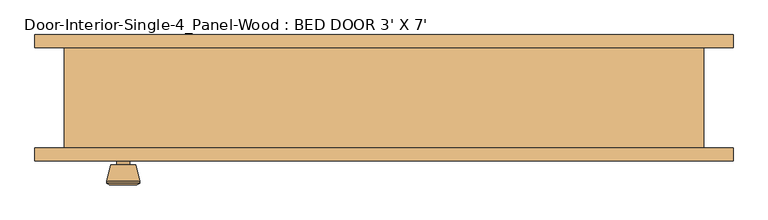
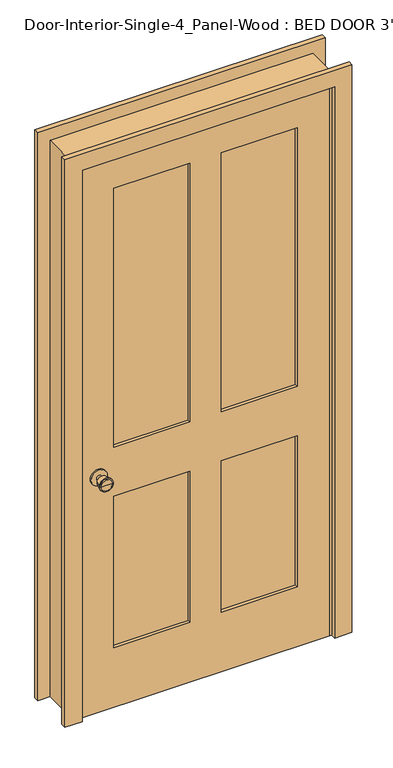
"""IFC4 building model written with IfcOpenShell, lengths in millimetres: door geometry, Door-Interior-Single-4_Panel-Wood : BED DOOR 3' X 7'."""

from ifc_helpers import new_model, si_unit, point, frame, frame_2d, origin, place, context, project, spatial, polyline, circle_curve, trimmed, segment, composite_curve, outline, extrude, faceted_brep, source, transform, mapped, element, save
from ifc_brep_helpers import plane_surface, cylinder_surface, revolved_surface, advanced_brep


def door_interior_single_4_panel_wood_bed_door_3_x_7_5a83478c(model_context):
    return source(origin(), model_context, "Body", "SolidModel", [
        advanced_brep(
        [(-393.7, -32.1, 914.4), (-403.7, -32.1, 914.4), (-383.7, -32.1, 914.4), (-373.2241324, 16.9, 914.4), (-414.1758676, 16.9, 914.4), (-393.7, 16.9, 914.4), (-368.7, 15.0721319, 914.4), (-418.7, 15.0721319, 914.4), (-368.7, 11.6084537, 914.4), (-418.7, 11.6084537, 914.4), (-375.063764, -13.1, 914.4), (-412.336236, -13.1, 914.4), (-383.7, -13.1, 914.4), (-403.7, -13.1, 914.4)],
        [
            (0, 1),
            (1, 2, circle_curve(frame((-393.7, -32.1, 914.4), z_axis=(0.0, -1.0, 0.0), x_axis=(-1.0, 0.0, 0.0)), 10.0)),
            (2, 0),
            (2, 1, circle_curve(frame((-393.7, -32.1, 914.4), z_axis=(0.0, -1.0, 0.0), x_axis=(-1.0, 0.0, 0.0)), 10.0)),
            (3, 4, circle_curve(frame((-393.7, 16.9, 914.4), z_axis=(0.0, 1.0, 0.0), x_axis=(-1.0, 0.0, 0.0)), 20.4758676)),
            (4, 5),
            (5, 3),
            (4, 3, circle_curve(frame((-393.7, 16.9, 914.4), z_axis=(0.0, 1.0, 0.0), x_axis=(-1.0, 0.0, 0.0)), 20.4758676)),
            (6, 7, circle_curve(frame((-393.7, 15.0721319, 914.4), z_axis=(0.0, 1.0, 0.0), x_axis=(-1.0, 0.0, 0.0)), 25.0)),
            (7, 4),
            (3, 6),
            (7, 6, circle_curve(frame((-393.7, 15.0721319, 914.4), z_axis=(0.0, 1.0, 0.0), x_axis=(-1.0, 0.0, 0.0)), 25.0)),
            (8, 9, circle_curve(frame((-393.7, 11.6084537, 914.4), z_axis=(0.0, 1.0, 0.0), x_axis=(-1.0, 0.0, 0.0)), 25.0)),
            (9, 7),
            (6, 8),
            (9, 8, circle_curve(frame((-393.7, 11.6084537, 914.4), z_axis=(0.0, 1.0, 0.0), x_axis=(-1.0, 0.0, 0.0)), 25.0)),
            (10, 11, circle_curve(frame((-393.7, -13.1, 914.4), z_axis=(0.0, 1.0, 0.0), x_axis=(-1.0, 0.0, 0.0)), 18.636236)),
            (11, 9),
            (8, 10),
            (11, 10, circle_curve(frame((-393.7, -13.1, 914.4), z_axis=(0.0, 1.0, 0.0), x_axis=(-1.0, 0.0, 0.0)), 18.636236)),
            (12, 13, circle_curve(frame((-393.7, -13.1, 914.4), z_axis=(0.0, 1.0, 0.0), x_axis=(-1.0, 0.0, 0.0)), 10.0)),
            (13, 11),
            (10, 12),
            (13, 12, circle_curve(frame((-393.7, -13.1, 914.4), z_axis=(0.0, 1.0, 0.0), x_axis=(-1.0, 0.0, 0.0)), 10.0)),
            (1, 13),
            (12, 2),
        ],
        [
            plane_surface(frame((-393.7, -32.1, 914.4), z_axis=(0.0, -1.0, 0.0), x_axis=(-1.0, 0.0, 0.0))),
            plane_surface(frame((-393.7, 16.9, 914.4), z_axis=(0.0, 1.0, 0.0), x_axis=(-1.0, 0.0, 0.0))),
            revolved_surface(polyline([(-414.1758676, 16.9, 914.4), (-418.7, 15.0721319, 914.4)]), (-393.7, -32.1, 914.4), (0.0, -1.0, 0.0)),
            cylinder_surface(frame((-393.7, -32.1, 914.4), z_axis=(0.0, -1.0, 0.0), x_axis=(-1.0, 0.0, 0.0)), 25.0),
            revolved_surface(polyline([(-418.7, 11.6084537, 914.4), (-412.336236, -13.1, 914.4)]), (-393.7, -32.1, 914.4), (0.0, -1.0, 0.0)),
            plane_surface(frame((-393.7, -13.1, 914.4), z_axis=(0.0, -1.0, 0.0), x_axis=(-1.0, 0.0, 0.0))),
            cylinder_surface(frame((-393.7, -32.1, 914.4), z_axis=(0.0, -1.0, 0.0), x_axis=(-1.0, 0.0, 0.0)), 10.0),
        ],
        [
            (0, [[1, 2, 3]]),
            (0, [[-3, 4, -1]]),
            (1, [[5, 6, 7]]),
            (1, [[8, -7, -6]]),
            (2, [[9, 10, -5, 11]]),
            (2, [[12, -11, -8, -10]]),
            (3, [[13, 14, -9, 15]]),
            (3, [[16, -15, -12, -14]]),
            (4, [[17, 18, -13, 19]]),
            (4, [[20, -19, -16, -18]]),
            (5, [[21, 22, -17, 23]]),
            (5, [[24, -23, -20, -22]]),
            (6, [[-2, 25, -21, 26]]),
            (6, [[-4, -26, -24, -25]]),
        ],
    ),
        extrude(outline(composite_curve([segment(trimmed(circle_curve(frame_2d((914.4, -393.7)), 30.0), [point((914.4, -423.7))], [point((914.4, -363.7))], False, "CARTESIAN"), True, "CONTINUOUS"), segment(trimmed(circle_curve(frame_2d((914.4, -393.7)), 30.0), [point((914.4, -363.7))], [point((914.4, -423.7))], False, "CARTESIAN"), True, "CONTINUOUS")], self_intersect=False)), frame((0.0, -38.1, 0.0), z_axis=(0.0, 1.0, 0.0), x_axis=(0.0, 0.0, 1.0)), (0.0, 0.0, 1.0), 6.0),
        advanced_brep(
        [(-393.7, -79.025, 914.4), (-383.7, -79.025, 914.4), (-403.7, -79.025, 914.4), (-373.2241324, -128.025, 914.4), (-393.7, -128.025, 914.4), (-414.1758676, -128.025, 914.4), (-368.7, -126.1971319, 914.4), (-418.7, -126.1971319, 914.4), (-368.7, -122.7334537, 914.4), (-418.7, -122.7334537, 914.4), (-375.063764, -98.025, 914.4), (-412.336236, -98.025, 914.4), (-383.7, -98.025, 914.4), (-403.7, -98.025, 914.4)],
        [
            (0, 1),
            (1, 2, circle_curve(frame((-393.7, -79.025, 914.4), z_axis=(0.0, 1.0, 0.0), x_axis=(-1.0, 0.0, 0.0)), 10.0)),
            (2, 0),
            (2, 1, circle_curve(frame((-393.7, -79.025, 914.4), z_axis=(0.0, 1.0, 0.0), x_axis=(-1.0, 0.0, 0.0)), 10.0)),
            (3, 4),
            (4, 5),
            (5, 3, circle_curve(frame((-393.7, -128.025, 914.4), z_axis=(0.0, -1.0, 0.0), x_axis=(-1.0, 0.0, 0.0)), 20.4758676)),
            (3, 5, circle_curve(frame((-393.7, -128.025, 914.4), z_axis=(0.0, -1.0, 0.0), x_axis=(-1.0, 0.0, 0.0)), 20.4758676)),
            (6, 3),
            (5, 7),
            (7, 6, circle_curve(frame((-393.7, -126.1971319, 914.4), z_axis=(0.0, -1.0, 0.0), x_axis=(-1.0, 0.0, 0.0)), 25.0)),
            (6, 7, circle_curve(frame((-393.7, -126.1971319, 914.4), z_axis=(0.0, -1.0, 0.0), x_axis=(-1.0, 0.0, 0.0)), 25.0)),
            (8, 6),
            (7, 9),
            (9, 8, circle_curve(frame((-393.7, -122.7334537, 914.4), z_axis=(0.0, -1.0, 0.0), x_axis=(-1.0, 0.0, 0.0)), 25.0)),
            (8, 9, circle_curve(frame((-393.7, -122.7334537, 914.4), z_axis=(0.0, -1.0, 0.0), x_axis=(-1.0, 0.0, 0.0)), 25.0)),
            (10, 8),
            (9, 11),
            (11, 10, circle_curve(frame((-393.7, -98.025, 914.4), z_axis=(0.0, -1.0, 0.0), x_axis=(-1.0, 0.0, 0.0)), 18.636236)),
            (10, 11, circle_curve(frame((-393.7, -98.025, 914.4), z_axis=(0.0, -1.0, 0.0), x_axis=(-1.0, 0.0, 0.0)), 18.636236)),
            (12, 10),
            (11, 13),
            (13, 12, circle_curve(frame((-393.7, -98.025, 914.4), z_axis=(0.0, -1.0, 0.0), x_axis=(-1.0, 0.0, 0.0)), 10.0)),
            (12, 13, circle_curve(frame((-393.7, -98.025, 914.4), z_axis=(0.0, -1.0, 0.0), x_axis=(-1.0, 0.0, 0.0)), 10.0)),
            (1, 12),
            (13, 2),
        ],
        [
            plane_surface(frame((-393.7, -79.025, 914.4), z_axis=(0.0, 1.0, 0.0), x_axis=(-1.0, 0.0, 0.0))),
            plane_surface(frame((-393.7, -128.025, 914.4), z_axis=(0.0, -1.0, 0.0), x_axis=(-1.0, 0.0, 0.0))),
            revolved_surface(polyline([(-414.1758676, -128.025, 914.4), (-418.7, -126.1971319, 914.4)]), (-393.7, -79.025, 914.4), (0.0, 1.0, 0.0)),
            cylinder_surface(frame((-393.7, -79.025, 914.4), z_axis=(0.0, 1.0, 0.0), x_axis=(-1.0, 0.0, 0.0)), 25.0),
            revolved_surface(polyline([(-418.7, -122.7334537, 914.4), (-412.336236, -98.025, 914.4)]), (-393.7, -79.025, 914.4), (0.0, 1.0, 0.0)),
            plane_surface(frame((-393.7, -98.025, 914.4), z_axis=(0.0, 1.0, 0.0), x_axis=(-1.0, 0.0, 0.0))),
            cylinder_surface(frame((-393.7, -79.025, 914.4), z_axis=(0.0, 1.0, 0.0), x_axis=(-1.0, 0.0, 0.0)), 10.0),
        ],
        [
            (0, [[1, 2, 3]]),
            (0, [[-3, 4, -1]]),
            (1, [[5, 6, 7]]),
            (1, [[-6, -5, 8]]),
            (2, [[9, -7, 10, 11]]),
            (2, [[-10, -8, -9, 12]]),
            (3, [[13, -11, 14, 15]]),
            (3, [[-14, -12, -13, 16]]),
            (4, [[17, -15, 18, 19]]),
            (4, [[-18, -16, -17, 20]]),
            (5, [[21, -19, 22, 23]]),
            (5, [[-22, -20, -21, 24]]),
            (6, [[25, -23, 26, -2]]),
            (6, [[-26, -24, -25, -4]]),
        ],
    ),
        extrude(outline(composite_curve([segment(trimmed(circle_curve(frame_2d((914.4, -393.7)), 30.0), [point((914.4, -423.7))], [point((914.4, -363.7))], False, "CARTESIAN"), True, "CONTINUOUS"), segment(trimmed(circle_curve(frame_2d((914.4, -393.7)), 30.0), [point((914.4, -363.7))], [point((914.4, -423.7))], False, "CARTESIAN"), True, "CONTINUOUS")], self_intersect=False)), frame((0.0, -79.025, 0.0), z_axis=(0.0, 1.0, 0.0), x_axis=(0.0, 0.0, 1.0)), (0.0, 0.0, 1.0), 6.0),
        faceted_brep([(482.6, -73.025, 0.0), (457.2, -73.025, 0.0), (457.2, -38.1, 0.0), (444.5, -38.1, 0.0), (444.5, -3.175, 0.0), (457.2, -3.175, 0.0), (457.2, 79.375, 0.0), (482.6, 79.375, 0.0), (482.6, 79.375, 2159.0), (482.6, -73.025, 2159.0), (457.2, 79.375, 2133.6), (-457.2, 79.375, 2133.6), (-457.2, 79.375, 0.0), (-482.6, 79.375, 0.0), (-482.6, 79.375, 2159.0), (457.2, -3.175, 2133.6), (444.5, -3.175, 2120.9), (-444.5, -3.175, 2120.9), (-444.5, -3.175, 0.0), (-457.2, -3.175, 0.0), (-457.2, -3.175, 2133.6), (444.5, -38.1, 2120.9), (457.2, -38.1, 2133.6), (-457.2, -38.1, 2133.6), (-457.2, -38.1, 0.0), (-444.5, -38.1, 0.0), (-444.5, -38.1, 2120.9), (457.2, -73.025, 2133.6), (-482.6, -73.025, 2159.0), (-482.6, -73.025, 0.0), (-457.2, -73.025, 0.0), (-457.2, -73.025, 2133.6)], [[[0, 1, 2, 3, 4, 5, 6, 7]], [[7, 8, 9, 0]], [[6, 10, 11, 12, 13, 14, 8, 7]], [[5, 15, 10, 6]], [[4, 16, 17, 18, 19, 20, 15, 5]], [[3, 21, 16, 4]], [[2, 22, 23, 24, 25, 26, 21, 3]], [[1, 27, 22, 2]], [[0, 9, 28, 29, 30, 31, 27, 1]], [[8, 14, 28, 9]], [[15, 20, 11, 10]], [[21, 26, 17, 16]], [[27, 31, 23, 22]], [[29, 13, 12, 19, 18, 25, 24, 30]], [[14, 13, 29, 28]], [[20, 19, 12, 11]], [[26, 25, 18, 17]], [[31, 30, 24, 23]]]),
        extrude(outline(polyline([(2133.6, -457.2), (0.0, -457.2), (0.0, 457.2), (2133.6, 457.2), (2133.6, -457.2)]), holes=[polyline([(2014.5375, 57.15), (2014.5375, 336.55), (1009.65, 336.55), (1009.65, 57.15), (2014.5375, 57.15)]), polyline([(1009.65, -57.15), (1009.65, -336.55), (2014.5375, -336.55), (2014.5375, -57.15), (1009.65, -57.15)]), polyline([(819.15, 57.15), (819.15, 336.55), (231.775, 336.55), (231.775, 57.15), (819.15, 57.15)]), polyline([(231.775, -57.15), (231.775, -336.55), (819.15, -336.55), (819.15, -57.15), (231.775, -57.15)])]), frame((0.0, -73.025, 0.0), z_axis=(0.0, 1.0, 0.0), x_axis=(0.0, 0.0, 1.0)), (0.0, 0.0, 1.0), 34.925),
        extrude(outline(polyline([(336.55, -49.7416667), (336.55, -61.3833333), (57.15, -61.3833333), (57.15, -49.7416667), (336.55, -49.7416667)])), frame((0.0, 0.0, 1009.65), z_axis=(0.0, 0.0, 1.0), x_axis=(1.0, 0.0, 0.0)), (0.0, 0.0, 1.0), 1004.8875),
        extrude(outline(polyline([(-57.15, -49.7416667), (-57.15, -61.3833333), (-336.55, -61.3833333), (-336.55, -49.7416667), (-57.15, -49.7416667)])), frame((0.0, 0.0, 1009.65), z_axis=(0.0, 0.0, 1.0), x_axis=(1.0, 0.0, 0.0)), (0.0, 0.0, 1.0), 1004.8875),
        extrude(outline(polyline([(336.55, -49.7416667), (336.55, -61.3833333), (57.15, -61.3833333), (57.15, -49.7416667), (336.55, -49.7416667)])), frame((0.0, 0.0, 231.775), z_axis=(0.0, 0.0, 1.0), x_axis=(1.0, 0.0, 0.0)), (0.0, 0.0, 1.0), 587.375),
        extrude(outline(polyline([(-57.15, -49.7416667), (-57.15, -61.3833333), (-336.55, -61.3833333), (-336.55, -49.7416667), (-57.15, -49.7416667)])), frame((0.0, 0.0, 231.775), z_axis=(0.0, 0.0, 1.0), x_axis=(1.0, 0.0, 0.0)), (0.0, 0.0, 1.0), 587.375),
        extrude(outline(polyline([(0.0, 527.05), (2203.45, 527.05), (2203.45, -527.05), (0.0, -527.05), (0.0, -463.55), (2139.95, -463.55), (2139.95, 463.55), (0.0, 463.55), (0.0, 527.05)])), frame((0.0, -92.075, 0.0), z_axis=(0.0, 1.0, 0.0), x_axis=(0.0, 0.0, 1.0)), (0.0, 0.0, 1.0), 19.05),
        extrude(outline(polyline([(0.0, 527.05), (2203.45, 527.05), (2203.45, -527.05), (0.0, -527.05), (0.0, -463.55), (2139.95, -463.55), (2139.95, 463.55), (0.0, 463.55), (0.0, 527.05)])), frame((0.0, 79.375, 0.0), z_axis=(0.0, 1.0, 0.0), x_axis=(0.0, 0.0, 1.0)), (0.0, 0.0, 1.0), 19.05),
    ])


if __name__ == "__main__":
    model = new_model("IFC4")
    model_context = context("Model", 3, world=origin())
    ifc_project = project(units=[si_unit("LENGTHUNIT", "METRE", prefix="MILLI")], contexts=[model_context])
    site = spatial("IfcSite", under=ifc_project)
    building = spatial("IfcBuilding", under=site)
    placement = place(None, origin())
    door_interior_single_4_panel_wood_bed_door_3_x_7_shape = door_interior_single_4_panel_wood_bed_door_3_x_7_5a83478c(model_context)
    element("IfcDoor", 1, ObjectType="Door-Interior-Single-4_Panel-Wood : BED DOOR 3' X 7'", at=placement, inside=building, context=model_context, shape_type="MappedRepresentation", body=[
        mapped(door_interior_single_4_panel_wood_bed_door_3_x_7_shape, transform((0.0, 0.0, 0.0), x_axis=(1.0, 0.0, 0.0), y_axis=(0.0, 1.0, 0.0), z_axis=(0.0, 0.0, 1.0))),
    ])
    save(model, "model.ifc")

# Revit data of these elements
# Type "Door-Interior-Single-4_Panel-Wood : BED DOOR 3' X 7'"
#   Type Mark = "13"
#   Assembly Code = "C1020300"
#   Analytic Construction = "Wooden"
#   Top Rail = 0' - 4 11/16"
#   Thickness = 0' - 1 3/8"
#   Thermal Resistance (R) = 2.5876 (h·ft²·°F)/BTU
#   Swing Angle [instance default] = 90.00°
#   Stiles = 0' - 4 3/4"
#   Rough Width = 3' - 2"
#   Rough Height = 7' - 1"
#   Mullion = 0' - 4 1/2"
#   Lock Rail = 0' - 7 1/2"
#   Height = 7' - 0"
#   Width = 3' - 0"
#   Heat Transfer Coefficient (U) = 0.3865 BTU/(h·ft²·°F)
#   Bottom Rail = 0' - 9 1/8"
#   Trim Material = Cherry
#   Panel Material = Cherry
#   Frame Material = Cherry
#   Door Handle Material = Aluminum
#   Visual Light Transmittance = 0
#   Solar Heat Gain Coefficient = 0
#   Wall Closure = (empty or 0)
#   Function = (empty or 0)
# Element 1 (IfcDoor, "Door-Interior-Single-4_Panel-Wood : BED DOOR 3' X 7'")
#   Materials on its faces: "Cherry", "Aluminum"
# Materials
#   "Cherry": class "Wood", colour RGB 226 177 128, transparency 0, Description = "Prunus Serotina", Cost = 0
#   "Aluminum": class "Metal", colour RGB 247 247 247, transparency 0, Description = "Aluminum 6061", Cost = 0
